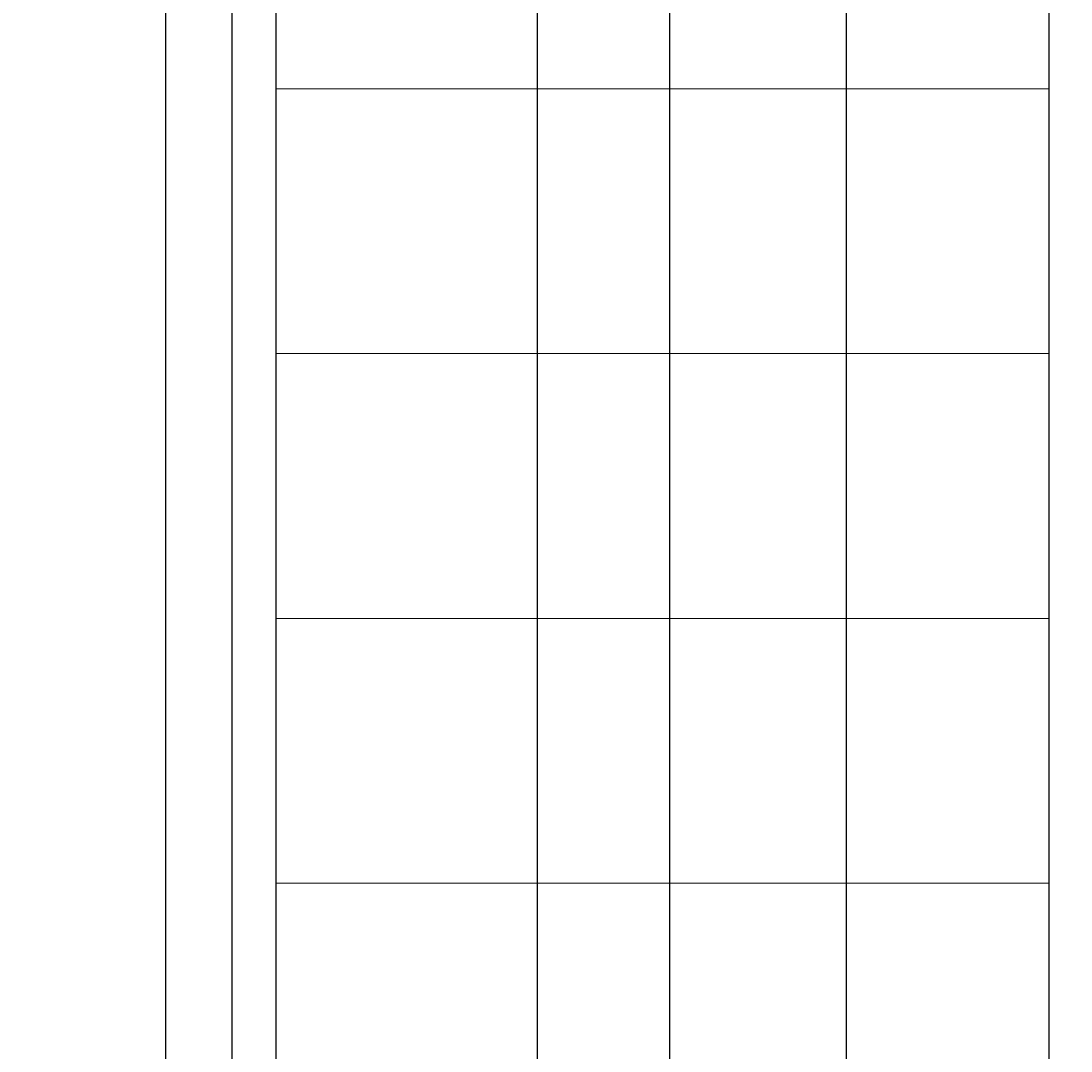
# Model space of a CAD drawing. Units: inches. Extents: x -6 to 289, y -8 to 323.
# Tile 57 of 107: x 124 to 147, y 182 to 206. Entities that reach past the tile are written whole.
import ezdxf

# ---------------------------------------------------------------- set-up
doc = ezdxf.new("R2010")
doc.units = ezdxf.units.IN
doc.header["$MEASUREMENT"] = 0
for name, color, linetype, lineweight in [('A-ANNO-DIMS', 2, 'Continuous', 18), ('A-ELEV-PATT', 8, 'Continuous', 13), ('A-GLAZ', 4, 'Continuous', 25)]:
    doc.layers.add(name, color=color, linetype=linetype, lineweight=lineweight)
doc.styles.get("Standard").update_dxf_attribs({"font": 'arial.ttf'})
doc.dimstyles.get("Standard").update_dxf_attribs({"dimtxt": 0.18, "dimasz": 0.18, "dimexe": 0.18, "dimexo": 0.0625, "dimgap": 0.09, "dimtad": 0, "dimtih": 1, "dimtoh": 1, "dimdec": 4, "dimzin": 0, "dimdsep": 46, "dimtxsty": 'Standard', "dimcen": 0.09, "dimadec": 0, "dimazin": 0, "dimtfac": 1, "dimtdec": 4, "dimtofl": 0, "dimtmove": 0, "dimatfit": 3, "dimfxl": 1, "dimtolj": 1, "dimtzin": 0, "dimarcsym": 0})

# ---------------------------------------------------------------- blocks, each defined once
blk = doc.blocks.new('*U4')
blk.add_line((1.5, 1.5), (1.5, 46.5))
blk.add_lwpolyline([(0, 0), (0, 48), (42, 48), (42, 0)], close=True)
blk.add_lwpolyline([(20, 45.5), (20, 2.5), (2.5, 2.5), (2.5, 45.5), (20, 45.5)])
blk = doc.blocks.new('*D25')
at = {"layer": 'A-ANNO-DIMS', "color": 0, "lineweight": -2, "transparency": 16777216}
for p, q in [((126.946, 226.654), (288.653, 226.654)), ((288.473, 226.474), (288.473, 202.836)), ((288.473, 178.834), (288.473, 202.472)), ((126.946, 178.654), (288.653, 178.654))]:
    blk.add_line(p, q, dxfattribs=at)
at = {"layer": 'A-ANNO-DIMS', "color": 0, "transparency": 16777216}
for points in [[(288.443, 226.474), (288.503, 226.474), (288.473, 226.654)], [(288.443, 178.834), (288.503, 178.834), (288.473, 178.654)]]:
    blk.add_solid(points, dxfattribs=at)
at = {"layer": 'Defpoints', "color": 0, "transparency": 16777216}
for p in [(126.883, 226.654), (288.473, 226.654), (126.883, 178.654)]:
    blk.add_point(p, dxfattribs=at)
at = {"layer": 'A-ANNO-DIMS', "color": 0, "transparency": 16777216, "insert": (288.473, 202.654), "char_height": 0.18, "attachment_point": 5}
blk.add_mtext('\\A1;48', dxfattribs=at)
blk = doc.blocks.new('*D73')
at = {"layer": 'A-ANNO-DIMS', "color": 0, "lineweight": -2, "transparency": 16777216}
for p, q in [((121.008, 51.148), (121.008, 322.969)), ((121.188, 322.789), (127.697, 322.789)), ((135.116, 322.789), (128.607, 322.789)), ((135.296, 51.148), (135.296, 322.969))]:
    blk.add_line(p, q, dxfattribs=at)
at = {"layer": 'A-ANNO-DIMS', "color": 0, "transparency": 16777216}
for points in [[(121.188, 322.819), (121.188, 322.759), (121.008, 322.789)], [(135.116, 322.819), (135.116, 322.759), (135.296, 322.789)]]:
    blk.add_solid(points, dxfattribs=at)
at = {"layer": 'Defpoints', "color": 0, "transparency": 16777216}
for p in [(135.296, 322.789), (121.008, 51.085), (135.296, 51.085)]:
    blk.add_point(p, dxfattribs=at)
at = {"layer": 'A-ANNO-DIMS', "color": 0, "transparency": 16777216, "insert": (128.152, 322.789), "char_height": 0.18, "attachment_point": 5}
blk.add_mtext('\\A1;14.288', dxfattribs=at)
blk = doc.blocks.new('*D74')
at = {"layer": 'A-ANNO-DIMS', "color": 0, "lineweight": -2, "transparency": 16777216}
for p, q in [((135.296, 51.148), (135.296, 322.969)), ((135.476, 322.789), (136.647, 322.789)), ((138.116, 322.789), (136.945, 322.789)), ((138.296, 51.148), (138.296, 322.969))]:
    blk.add_line(p, q, dxfattribs=at)
at = {"layer": 'A-ANNO-DIMS', "color": 0, "transparency": 16777216}
for points in [[(135.476, 322.819), (135.476, 322.759), (135.296, 322.789)], [(138.116, 322.819), (138.116, 322.759), (138.296, 322.789)]]:
    blk.add_solid(points, dxfattribs=at)
at = {"layer": 'Defpoints', "color": 0, "transparency": 16777216}
for p in [(138.296, 322.789), (135.296, 51.085), (138.296, 51.085)]:
    blk.add_point(p, dxfattribs=at)
at = {"layer": 'A-ANNO-DIMS', "color": 0, "transparency": 16777216, "insert": (136.796, 322.789), "char_height": 0.18, "attachment_point": 5}
blk.add_mtext('\\A1;3', dxfattribs=at)
blk = doc.blocks.new('*D75')
at = {"layer": 'A-ANNO-DIMS', "color": 0, "lineweight": -2, "transparency": 16777216}
for p, q in [((138.296, 51.148), (138.296, 322.969)), ((138.476, 322.789), (140.144, 322.789)), ((142.116, 322.789), (140.448, 322.789)), ((142.296, 51.148), (142.296, 322.969))]:
    blk.add_line(p, q, dxfattribs=at)
at = {"layer": 'A-ANNO-DIMS', "color": 0, "transparency": 16777216}
for points in [[(138.476, 322.819), (138.476, 322.759), (138.296, 322.789)], [(142.116, 322.819), (142.116, 322.759), (142.296, 322.789)]]:
    blk.add_solid(points, dxfattribs=at)
at = {"layer": 'Defpoints', "color": 0, "transparency": 16777216}
for p in [(142.296, 322.789), (138.296, 51.085), (142.296, 51.085)]:
    blk.add_point(p, dxfattribs=at)
at = {"layer": 'A-ANNO-DIMS', "color": 0, "transparency": 16777216, "insert": (140.296, 322.789), "char_height": 0.18, "attachment_point": 5}
blk.add_mtext('\\A1;4', dxfattribs=at)
blk = doc.blocks.new('*D76')
at = {"layer": 'A-ANNO-DIMS', "color": 0, "lineweight": -2, "transparency": 16777216}
for p, q in [((142.296, 51.148), (142.296, 322.969)), ((142.476, 322.789), (153.076, 322.789)), ((164.116, 322.789), (153.516, 322.789)), ((164.296, 51.148), (164.296, 322.969))]:
    blk.add_line(p, q, dxfattribs=at)
at = {"layer": 'A-ANNO-DIMS', "color": 0, "transparency": 16777216}
for points in [[(142.476, 322.819), (142.476, 322.759), (142.296, 322.789)], [(164.116, 322.819), (164.116, 322.759), (164.296, 322.789)]]:
    blk.add_solid(points, dxfattribs=at)
at = {"layer": 'Defpoints', "color": 0, "transparency": 16777216}
for p in [(164.296, 322.789), (142.296, 51.085), (164.296, 51.085)]:
    blk.add_point(p, dxfattribs=at)
at = {"layer": 'A-ANNO-DIMS', "color": 0, "transparency": 16777216, "insert": (153.296, 322.789), "char_height": 0.18, "attachment_point": 5}
blk.add_mtext('\\A1;22', dxfattribs=at)
blk = doc.blocks.new('*D94')
at = {"layer": 'A-ANNO-DIMS', "color": 0, "lineweight": -2, "transparency": 16777216}
for p, q in [((118.164, 159.411), (118.164, 322.969)), ((118.344, 322.789), (139.46, 322.789)), ((161.372, 322.789), (140.256, 322.789)), ((161.552, 159.411), (161.552, 322.969))]:
    blk.add_line(p, q, dxfattribs=at)
at = {"layer": 'A-ANNO-DIMS', "color": 0, "transparency": 16777216}
for points in [[(118.344, 322.819), (118.344, 322.759), (118.164, 322.789)], [(161.372, 322.819), (161.372, 322.759), (161.552, 322.789)]]:
    blk.add_solid(points, dxfattribs=at)
at = {"layer": 'Defpoints', "color": 0, "transparency": 16777216}
for p in [(161.552, 322.789), (118.164, 159.348), (161.552, 159.348)]:
    blk.add_point(p, dxfattribs=at)
at = {"layer": 'A-ANNO-DIMS', "color": 0, "transparency": 16777216, "insert": (139.858, 322.789), "char_height": 0.18, "attachment_point": 5}
blk.add_mtext('\\A1;43.39', dxfattribs=at)

msp = doc.modelspace()

# ---------------------------------------------------------------- hatches: boundary and pattern name
at = {"layer": 'A-ELEV-PATT'}
h = msp.add_hatch(dxfattribs=at)
h.set_pattern_fill('_USER', color=256, scale=6, pattern_type=0)
h.set_pattern_definition([(0, (0, 0), (0, 6), [])])
h.paths.add_polyline_path([(184.1244, 48.0851), (124.008, 48.0851), (124.008, 10.2888), (184.1244, 10.2888)])
h.paths.add_polyline_path([(244.2408, 48.0851), (186.3604, 48.0851), (186.3604, 10.2888), (244.2408, 10.2888)])
h.paths.add_polyline_path([(208.2918, 114.2795), (190.7918, 114.2795), (190.7918, 71.2795), (208.2918, 71.2795)])
h.paths.add_polyline_path([(227.7918, 114.2795), (209.2918, 114.2795), (209.2918, 71.2795), (227.7918, 71.2795)])
h.paths.add_polyline_path([(211.2918, 224.3887), (190.7918, 224.3887), (190.7918, 162.3484), (211.2918, 162.3484)])
h.paths.add_polyline_path([(233.7918, 224.3887), (212.2918, 224.3887), (212.2918, 162.3484), (233.7918, 162.3484)])
h.paths.add_polyline_path([(166.3835, 224.154), (147.8835, 224.154), (147.8835, 181.154), (166.3835, 181.154)])
h.paths.add_polyline_path([(146.8835, 224.154), (129.3835, 224.154), (129.3835, 181.154), (146.8835, 181.154)])

# ---------------------------------------------------------------- block references
at = {"layer": 'A-GLAZ'}
msp.add_blockref('*U4', (126.8835, 178.654), dxfattribs=at)

# ---------------------------------------------------------------- dimensions: what is measured, and where the dimension line sits
at = {"layer": 'A-ANNO-DIMS'}
for base, p1, p2, override, picture, middle in [((161.5522, 322.7888), (118.1638, 159.3484), (161.5522, 159.3484), {"dimdec": 2, "dimlfac": 1, "dimrnd": 0, "dimzin": 0, "dimdsep": 46, "dimlunit": 2}, '*D94', (139.858, 322.7888)), ((135.296, 322.7888), (121.008, 51.0851), (135.296, 51.0851), {"dimdec": 3, "dimlfac": 1, "dimrnd": 0, "dimzin": 0, "dimdsep": 46, "dimlunit": 2}, '*D73', (128.152, 322.7888)), ((138.296, 322.7888), (135.296, 51.0851), (138.296, 51.0851), {"dimdec": 0, "dimlfac": 1, "dimrnd": 0, "dimzin": 0, "dimdsep": 46, "dimlunit": 2}, '*D74', (136.796, 322.7888)), ((142.296, 322.7888), (138.296, 51.0851), (142.296, 51.0851), {"dimdec": 0, "dimlfac": 1, "dimrnd": 0, "dimzin": 0, "dimdsep": 46, "dimlunit": 2}, '*D75', (140.296, 322.7888)), ((164.296, 322.7888), (142.296, 51.0851), (164.296, 51.0851), {"dimdec": 0, "dimlfac": 1, "dimrnd": 0, "dimzin": 0, "dimdsep": 46, "dimlunit": 2}, '*D76', (153.296, 322.7888))]:
    dim = msp.add_linear_dim(base=base, p1=p1, p2=p2, dimstyle='Standard', override=override, dxfattribs=at)
    dim.commit()
    dim.dimension.update_dxf_attribs({"geometry": picture, "text_midpoint": middle})
dim = msp.add_linear_dim(base=(288.4733, 226.654), p1=(126.8835, 178.654), p2=(126.8835, 226.654), angle=90, dimstyle='Standard', override={"dimdec": 0, "dimlfac": 1, "dimrnd": 0, "dimzin": 0, "dimdsep": 46, "dimlunit": 2}, dxfattribs=at)
dim.commit()
dim.dimension.update_dxf_attribs({"geometry": '*D25', "text_midpoint": (288.4733, 202.654)})

doc.saveas('drawing.dxf')
